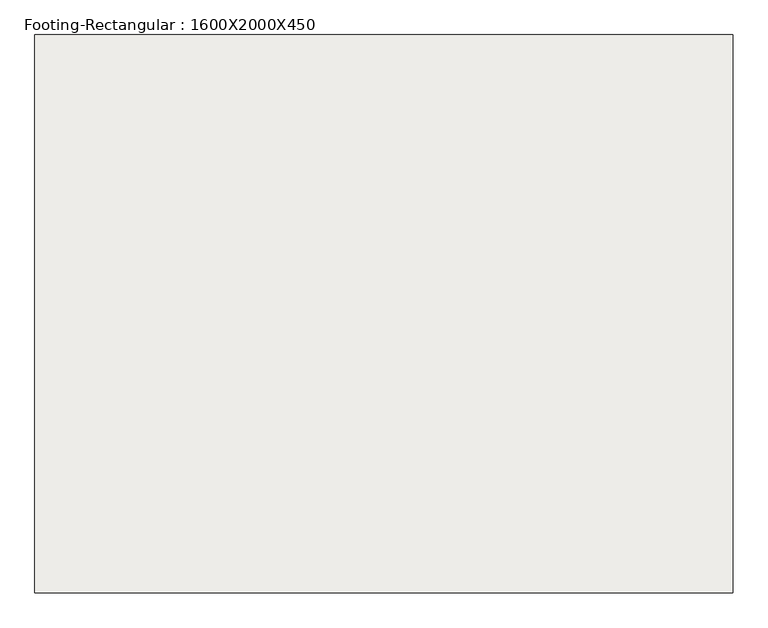
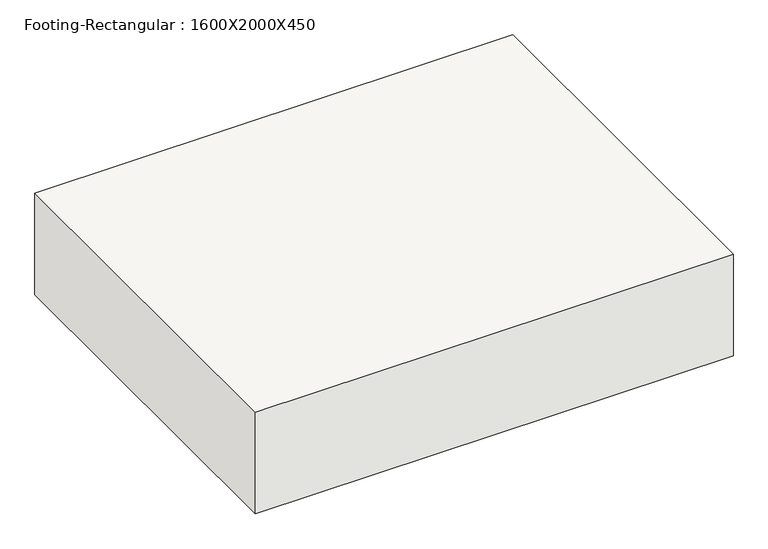
"""IFC4 building model written with IfcOpenShell, lengths in millimetres: slab geometry, Footing-Rectangular : 1600X2000X450."""

from ifc_helpers import new_model, si_unit, frame, origin, place, context, project, spatial, polyline, outline, extrude, source, transform, mapped, element, save


def footing_rectangular_1600x2000x450_9a9f7728(model_context):
    return source(origin(), model_context, "Body", "SweptSolid", [
        extrude(outline(polyline([(1000.0, 800.0), (1000.0, -800.0), (-1000.0, -800.0), (-1000.0, 800.0), (1000.0, 800.0)])), frame((0.0, 0.0, -450.0), z_axis=(0.0, 0.0, 1.0), x_axis=(1.0, 0.0, 0.0)), (0.0, 0.0, 1.0), 450.0),
    ])


if __name__ == "__main__":
    model = new_model("IFC4")
    model_context = context("Model", 3, world=origin())
    ifc_project = project(units=[si_unit("LENGTHUNIT", "METRE", prefix="MILLI")], contexts=[model_context])
    site = spatial("IfcSite", under=ifc_project)
    building = spatial("IfcBuilding", under=site)
    placement = place(None, origin())
    footing_rectangular_1600x2000x450_shape = footing_rectangular_1600x2000x450_9a9f7728(model_context)
    element("IfcSlab", 1, ObjectType="Footing-Rectangular : 1600X2000X450", at=placement, inside=building, context=model_context, shape_type="MappedRepresentation", body=[
        mapped(footing_rectangular_1600x2000x450_shape, transform((0.0, 0.0, 0.0), x_axis=(1.0, 0.0, 0.0), y_axis=(0.0, 1.0, 0.0), z_axis=(0.0, 0.0, 1.0))),
    ])
    save(model, "model.ifc")

# Revit data of these elements
# Type "Footing-Rectangular : 1600X2000X450"
#   Width = 6' - 6.74016"
#   Length = 5' - 2.99213"
#   Foundation Thickness = 1' - 5.71654"
#   Structural Material [instance default] = Concrete - Cast-in-Place Concrete
#   Assembly Code = ""
# Element 1 (IfcSlab, "Footing-Rectangular : 1600X2000X450")
#   Materials on its faces: "Concrete - Cast-in-Place Concrete"
# Materials
#   "Concrete - Cast-in-Place Concrete": class "Concrete", colour RGB 192 192 192, transparency 0, Cost = 0
